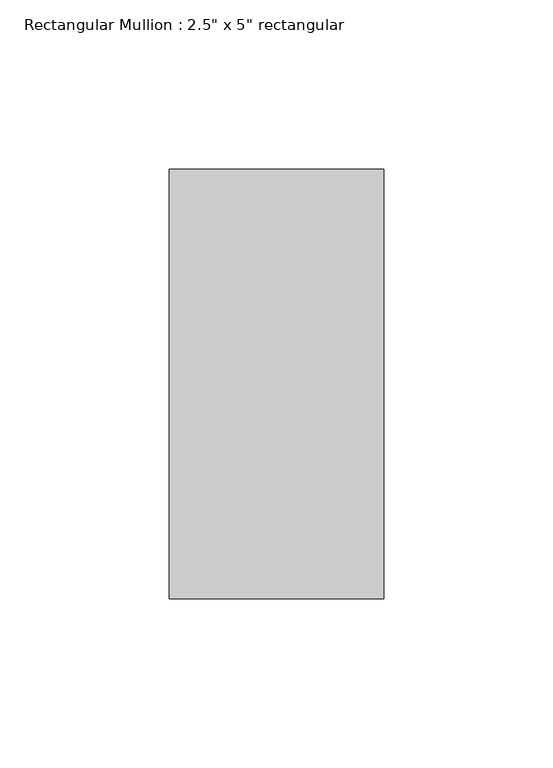
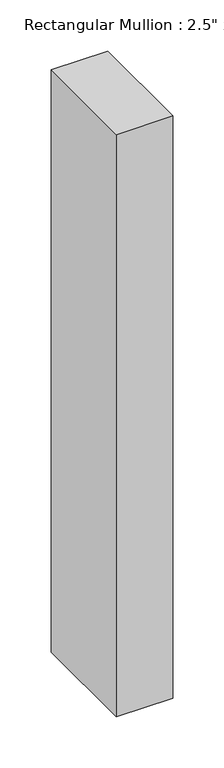
"""IFC4 building model written with IfcOpenShell, lengths in millimetres: member geometry."""

from ifc_helpers import new_model, si_unit, frame, origin, place, context, project, spatial, polyline, outline, extrude, source, transform, mapped, element, save


def member_48a7c542(model_context):
    return source(origin(), model_context, "Body", "SweptSolid", [
        extrude(outline(polyline([(0.0, 63.5), (0.0, -63.5), (-63.5, -63.5), (-63.5, 63.5), (0.0, 63.5)])), frame((0.0, 0.0, -693.4021067), z_axis=(0.0, 0.0, 1.0), x_axis=(1.0, 0.0, 0.0)), (0.0, 0.0, 1.0), 693.4021067),
    ])


if __name__ == "__main__":
    model = new_model("IFC4")
    model_context = context("Model", 3, world=origin())
    ifc_project = project(units=[si_unit("LENGTHUNIT", "METRE", prefix="MILLI")], contexts=[model_context])
    site = spatial("IfcSite", under=ifc_project)
    building = spatial("IfcBuilding", under=site)
    placement = place(None, origin())
    member_shape = member_48a7c542(model_context)
    element("IfcMember", 1, ObjectType="Rectangular Mullion : 2.5\" x 5\" rectangular", at=placement, inside=building, context=model_context, shape_type="MappedRepresentation", body=[
        mapped(member_shape, transform((0.0, 0.0, 0.0), x_axis=(1.0, 0.0, 0.0), y_axis=(0.0, 1.0, 0.0), z_axis=(0.0, 0.0, 1.0))),
    ])
    save(model, "model.ifc")

# Revit data of these elements
# Type "Rectangular Mullion : 2.5\" x 5\" rectangular"
#   built-in parameter 1007304 = 0.416667 (stored number, unit not read)
#   built-in parameter 1007301 = 0.104167 (stored number, unit not read)
#   built-in parameter 1007300 = 0.104167 (stored number, unit not read)
# Element 1 (IfcMember, "Rectangular Mullion : 2.5\" x 5\" rectangular")
#   Materials on its faces: "Aluminum"
# Materials
#   "Aluminum": class "Metal", colour RGB 247 247 247, transparency 0, Description = "Aluminum 6061", Cost = 0
